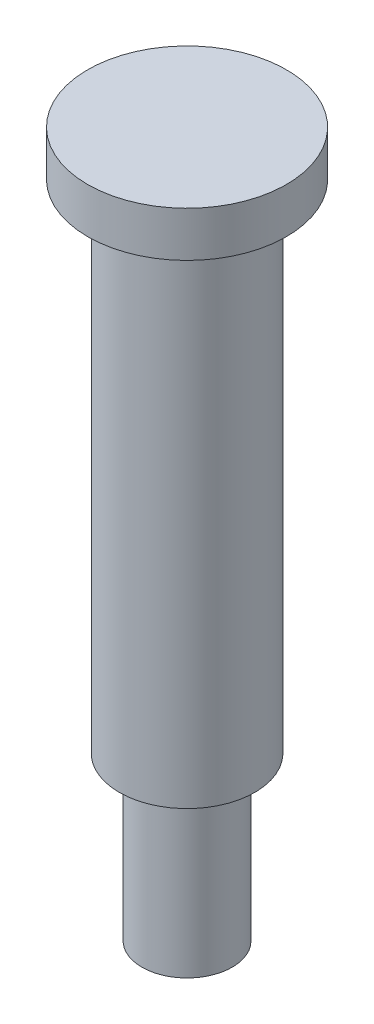
ISO-10303-21;
HEADER;
FILE_DESCRIPTION(('STEP AP214'),'2;1');
FILE_NAME('part.step','',(''),(''),'','','');
FILE_SCHEMA(('AUTOMOTIVE_DESIGN { 1 0 10303 214 1 1 1 1 }'));
ENDSEC;
DATA;
#1=APPLICATION_CONTEXT('core data for automotive mechanical design processes');
#2=APPLICATION_PROTOCOL_DEFINITION('international standard','automotive_design',2000,#1);
#3=PRODUCT_CONTEXT('',#1,'mechanical');
#4=PRODUCT('Part','Part','',(#3));
#5=PRODUCT_RELATED_PRODUCT_CATEGORY('part','',(#4));
#6=PRODUCT_DEFINITION_FORMATION('','',#4);
#7=PRODUCT_DEFINITION_CONTEXT('part definition',#1,'design');
#8=PRODUCT_DEFINITION('design','',#6,#7);
#9=PRODUCT_DEFINITION_SHAPE('','',#8);
#10=(LENGTH_UNIT() NAMED_UNIT(*) SI_UNIT(.MILLI.,.METRE.));
#11=(NAMED_UNIT(*) PLANE_ANGLE_UNIT() SI_UNIT($,.RADIAN.));
#12=(NAMED_UNIT(*) SI_UNIT($,.STERADIAN.) SOLID_ANGLE_UNIT());
#13=UNCERTAINTY_MEASURE_WITH_UNIT(LENGTH_MEASURE(1.E-05),#10,'distance_accuracy_value','');
#14=(GEOMETRIC_REPRESENTATION_CONTEXT(3) GLOBAL_UNCERTAINTY_ASSIGNED_CONTEXT((#13)) GLOBAL_UNIT_ASSIGNED_CONTEXT((#10,
#11,#12)) REPRESENTATION_CONTEXT('',''));
#15=CARTESIAN_POINT('',(0.,0.,0.));
#16=DIRECTION('',(0.,0.,1.));
#17=DIRECTION('',(1.,0.,0.));
#18=AXIS2_PLACEMENT_3D('',#15,#16,#17);
#19=CARTESIAN_POINT('',(0.,0.,0.));
#20=DIRECTION('',(0.,1.,0.));
#21=DIRECTION('',(0.,0.,1.));
#22=AXIS2_PLACEMENT_3D('',#19,#20,#21);
#23=PLANE('',#22);
#24=CARTESIAN_POINT('',(0.,0.,0.));
#25=DIRECTION('',(0.,1.,0.));
#26=DIRECTION('',(0.,0.,1.));
#27=AXIS2_PLACEMENT_3D('',#24,#25,#26);
#28=CIRCLE('',#27,11.);
#29=CARTESIAN_POINT('',(0.,0.,11.));
#30=VERTEX_POINT('',#29);
#31=EDGE_CURVE('E10',#30,#30,#28,.T.);
#32=ORIENTED_EDGE('',*,*,#31,.T.);
#33=EDGE_LOOP('',(#32));
#34=FACE_BOUND('',#33,.T.);
#35=ADVANCED_FACE('F40',(#34),#23,.T.);
#36=CARTESIAN_POINT('',(0.,16.2432432432432,0.));
#37=DIRECTION('',(0.,1.,0.));
#38=DIRECTION('',(0.,0.,1.));
#39=AXIS2_PLACEMENT_3D('',#36,#37,#38);
#40=CYLINDRICAL_SURFACE('',#39,11.);
#41=CARTESIAN_POINT('',(0.,-5.,0.));
#42=DIRECTION('',(0.,1.,0.));
#43=DIRECTION('',(0.,0.,1.));
#44=AXIS2_PLACEMENT_3D('',#41,#42,#43);
#45=CIRCLE('',#44,11.);
#46=CARTESIAN_POINT('',(0.,-5.,11.));
#47=VERTEX_POINT('',#46);
#48=EDGE_CURVE('E43',#47,#47,#45,.T.);
#49=ORIENTED_EDGE('',*,*,#48,.T.);
#50=EDGE_LOOP('',(#49));
#51=FACE_BOUND('',#50,.T.);
#52=ORIENTED_EDGE('',*,*,#31,.F.);
#53=EDGE_LOOP('',(#52));
#54=FACE_BOUND('',#53,.T.);
#55=ADVANCED_FACE('F73',(#51,#54),#40,.T.);
#56=CARTESIAN_POINT('',(-11.,-5.,0.));
#57=DIRECTION('',(0.,-1.,0.));
#58=DIRECTION('',(0.,0.,-1.));
#59=AXIS2_PLACEMENT_3D('',#56,#57,#58);
#60=PLANE('',#59);
#61=CARTESIAN_POINT('',(0.,-5.,0.));
#62=DIRECTION('',(0.,1.,0.));
#63=DIRECTION('',(0.,0.,1.));
#64=AXIS2_PLACEMENT_3D('',#61,#62,#63);
#65=CIRCLE('',#64,7.5);
#66=CARTESIAN_POINT('',(0.,-5.,7.5));
#67=VERTEX_POINT('',#66);
#68=EDGE_CURVE('E50',#67,#67,#65,.T.);
#69=ORIENTED_EDGE('',*,*,#68,.T.);
#70=EDGE_LOOP('',(#69));
#71=FACE_BOUND('',#70,.T.);
#72=ORIENTED_EDGE('',*,*,#48,.F.);
#73=EDGE_LOOP('',(#72));
#74=FACE_BOUND('',#73,.T.);
#75=ADVANCED_FACE('F79',(#71,#74),#60,.T.);
#76=CARTESIAN_POINT('',(0.,16.2432432432432,0.));
#77=DIRECTION('',(0.,1.,0.));
#78=DIRECTION('',(0.,0.,1.));
#79=AXIS2_PLACEMENT_3D('',#76,#77,#78);
#80=CYLINDRICAL_SURFACE('',#79,7.49999999999999);
#81=CARTESIAN_POINT('',(0.,-60.,0.));
#82=DIRECTION('',(0.,1.,0.));
#83=DIRECTION('',(0.,0.,1.));
#84=AXIS2_PLACEMENT_3D('',#81,#82,#83);
#85=CIRCLE('',#84,7.49999999999999);
#86=CARTESIAN_POINT('',(0.,-60.,7.49999999999999));
#87=VERTEX_POINT('',#86);
#88=EDGE_CURVE('E51',#87,#87,#85,.T.);
#89=ORIENTED_EDGE('',*,*,#88,.T.);
#90=EDGE_LOOP('',(#89));
#91=FACE_BOUND('',#90,.T.);
#92=ORIENTED_EDGE('',*,*,#68,.F.);
#93=EDGE_LOOP('',(#92));
#94=FACE_BOUND('',#93,.T.);
#95=ADVANCED_FACE('F84',(#91,#94),#80,.T.);
#96=CARTESIAN_POINT('',(-7.49999999999999,-60.,0.));
#97=DIRECTION('',(0.,-1.,0.));
#98=DIRECTION('',(0.,0.,-1.));
#99=AXIS2_PLACEMENT_3D('',#96,#97,#98);
#100=PLANE('',#99);
#101=CARTESIAN_POINT('',(0.,-60.,0.));
#102=DIRECTION('',(0.,1.,0.));
#103=DIRECTION('',(0.,0.,1.));
#104=AXIS2_PLACEMENT_3D('',#101,#102,#103);
#105=CIRCLE('',#104,4.99999999999999);
#106=CARTESIAN_POINT('',(0.,-60.,4.99999999999999));
#107=VERTEX_POINT('',#106);
#108=EDGE_CURVE('E57',#107,#107,#105,.T.);
#109=ORIENTED_EDGE('',*,*,#108,.T.);
#110=EDGE_LOOP('',(#109));
#111=FACE_BOUND('',#110,.T.);
#112=ORIENTED_EDGE('',*,*,#88,.F.);
#113=EDGE_LOOP('',(#112));
#114=FACE_BOUND('',#113,.T.);
#115=ADVANCED_FACE('F75',(#111,#114),#100,.T.);
#116=CARTESIAN_POINT('',(0.,16.2432432432432,0.));
#117=DIRECTION('',(0.,1.,0.));
#118=DIRECTION('',(0.,0.,1.));
#119=AXIS2_PLACEMENT_3D('',#116,#117,#118);
#120=CYLINDRICAL_SURFACE('',#119,4.99999999999999);
#121=CARTESIAN_POINT('',(0.,-78.,0.));
#122=DIRECTION('',(0.,1.,0.));
#123=DIRECTION('',(0.,0.,1.));
#124=AXIS2_PLACEMENT_3D('',#121,#122,#123);
#125=CIRCLE('',#124,4.99999999999999);
#126=CARTESIAN_POINT('',(0.,-78.,4.99999999999999));
#127=VERTEX_POINT('',#126);
#128=EDGE_CURVE('E56',#127,#127,#125,.T.);
#129=ORIENTED_EDGE('',*,*,#128,.T.);
#130=EDGE_LOOP('',(#129));
#131=FACE_BOUND('',#130,.T.);
#132=ORIENTED_EDGE('',*,*,#108,.F.);
#133=EDGE_LOOP('',(#132));
#134=FACE_BOUND('',#133,.T.);
#135=ADVANCED_FACE('F61',(#131,#134),#120,.T.);
#136=CARTESIAN_POINT('',(-4.99999999999999,-78.,0.));
#137=DIRECTION('',(0.,-1.,0.));
#138=DIRECTION('',(0.,0.,-1.));
#139=AXIS2_PLACEMENT_3D('',#136,#137,#138);
#140=PLANE('',#139);
#141=ORIENTED_EDGE('',*,*,#128,.F.);
#142=EDGE_LOOP('',(#141));
#143=FACE_BOUND('',#142,.T.);
#144=ADVANCED_FACE('F66',(#143),#140,.T.);
#145=CLOSED_SHELL('',(#35,#55,#75,#95,#115,#135,#144));
#146=MANIFOLD_SOLID_BREP('B2',#145);
#147=ADVANCED_BREP_SHAPE_REPRESENTATION('',(#18,#146),#14);
#148=SHAPE_DEFINITION_REPRESENTATION(#9,#147);
ENDSEC;
END-ISO-10303-21;
